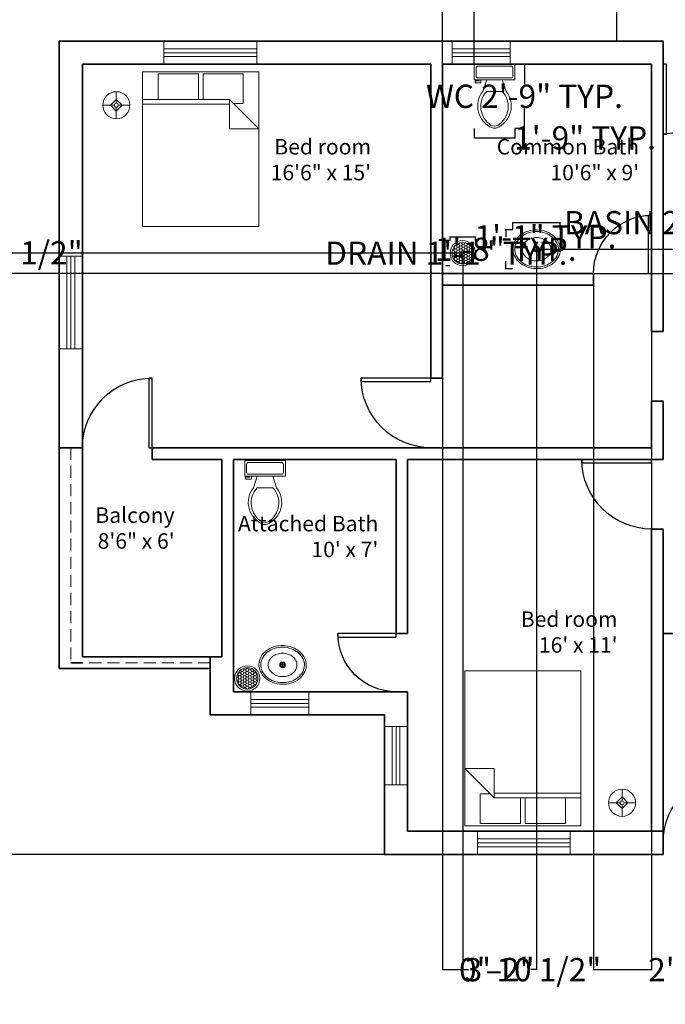
# Model space of a CAD drawing. Units: inches. Extents: x 2450 to 4494, y 1482 to 2597.
# Tile 4 of 7: x 3238 to 3571, y 1482 to 1990. Entities that reach past the tile are written whole.
import ezdxf

# ---------------------------------------------------------------- set-up
doc = ezdxf.new("R2010")
doc.units = ezdxf.units.IN
doc.header["$LTSCALE"] = 5
doc.header["$MEASUREMENT"] = 0
doc.linetypes.add('HIDDEN', pattern=[0.375, 0.25, -0.125])
for name, color, linetype, lineweight in [('A-ANNO-DIMS', 2, 'Continuous', 18), ('A-AREA-IDEN', 7, 'Continuous', 18), ('A-DOOR', 4, 'Continuous', 25), ('A-FLOR-EDGE', 7, 'Continuous', 25), ('A-FLOR-FIXT', 9, 'Continuous', 18), ('A-FURN', 8, 'Continuous', 18), ('A-GLAZ', 4, 'Continuous', 18), ('A-WALL', 7, 'Continuous', 35), ('A-WALL-HIDN', 7, 'HIDDEN', 18)]:
    doc.layers.add(name, color=color, linetype=linetype, lineweight=lineweight)
doc.styles.get("Standard").update_dxf_attribs({"font": 'arial.ttf'})
doc.dimstyles.get("Standard").update_dxf_attribs({"dimtxt": 12, "dimasz": 0.18, "dimexe": 0.18, "dimexo": 0.0625, "dimgap": 0.09, "dimtad": 0, "dimtih": 1, "dimtoh": 1, "dimdec": 0, "dimzin": 0, "dimdsep": 46, "dimlunit": 3, "dimtxsty": 'Standard', "dimcen": 0.09, "dimadec": 0, "dimazin": 0, "dimtfac": 1, "dimtdec": 0, "dimtofl": 0, "dimtmove": 0, "dimatfit": 3, "dimfxl": 1, "dimtolj": 1, "dimtzin": 0, "dimarcsym": 0})

# ---------------------------------------------------------------- blocks, each defined once
blk = doc.blocks.new('*U2')
for p, q in [((0, 0), (0, -6)), ((36, 0), (36, -6))]:
    blk.add_line(p, q)
blk.add_lwpolyline([(0, 0), (0, 36), (1.75, 36), (1.75, 0)], close=True)
blk.add_arc((0, 0), 36, 0, 90)
blk = doc.blocks.new('*U3')
for p, q in [((0, 0), (0, -6)), ((30, 0), (30, -6))]:
    blk.add_line(p, q)
blk.add_lwpolyline([(0, 0), (0, 30), (1.75, 30), (1.75, 0)], close=True)
blk.add_arc((0, 0), 30, 0, 90)
blk = doc.blocks.new('*U5')
for p, q in [((-36, 0), (-36, 6)), ((0, 0), (0, 6))]:
    blk.add_line(p, q)
blk.add_lwpolyline([(0, 0), (0, -36), (-1.75, -36), (-1.75, 0)], close=True)
blk.add_arc((0, 0), 36, 180, 270)
blk = doc.blocks.new('Bed - Queen')
for p, q in [((0, -80.00003), (0, 0)), ((0, 0), (59.99999, 0)), ((59.99999, 0), (59.99999, -80.00003)), ((7.99999, -1.2), (28.79998, -1.2)), ((7.99999, -14.4), (7.99999, -1.2)), ((28.79998, -1.2), (28.79998, -14.4)), ((31.19999, -1.2), (51.99999, -1.2)), ((31.19999, -14.4), (31.19999, -1.2)), ((51.99999, -1.2), (51.99999, -16.4)), ((0, -14.4), (44.8, -14.4)), ((59.99999, -29.6), (44.8, -14.4)), ((44.8, -14.4), (44.8, -29.6)), ((44.8, -16.8), (0, -16.8)), ((51.99999, -16.4), (46.79936, -16.4)), ((44.8, -29.6), (59.99999, -29.6)), ((59.99999, -80.00003), (0, -80.00003))]:
    blk.add_line(p, q)
blk = doc.blocks.new('Lamp - Table')
for p, q in [((0, 7), (0, 1)), ((-1, 0), (-7, 0)), ((0, 3), (-3, 0)), ((-3, 0), (0, -3)), ((3, 0), (0, 3)), ((0, -3), (3, 0)), ((1, 0), (7, 0)), ((0, -1), (0, -7))]:
    blk.add_line(p, q)
for radius in [7, 1]:
    blk.add_circle((0, 0), radius)
blk = doc.blocks.new('Toilet - top')
for p, q in [((9.5, -6), (9.5, -2)), ((-10, -8.5), (-8, -8.5)), ((-10, -9.5), (-10, -8.5)), ((-7, -9.5), (-10, -9.5)), ((-8, -8.5), (-8, -8)), ((-7, -8), (-7, -9.5)), ((-4, -8), (-6, -14)), ((4, -8), (6, -14)), ((4, -14), (-4, -14))]:
    blk.add_line(p, q)
blk.add_lwpolyline([(10.5, -8), (10.5, 0), (-10.5, 0), (-10.5, -8)], close=True)
for points in [[(-9.5, -2), (-9.5, -6)], [(8.5, -1), (-8.5, -1)], [(-8.5, -7), (8.5, -7)]]:
    blk.add_lwpolyline(points)
for centre, radius, start, end in [((-8.62, -1.88), 0.884, 81.8699, 188.1301), ((8.62, -1.88), 0.884, 351.8699, 98.1301), ((-8.62, -6.12), 0.884, 171.8699, 278.1301), ((8.62, -6.12), 0.884, 261.8699, 8.1301), ((3.52, -21.58), 12.17, 141.4691, 247.9714), ((4.2, -21.82), 11.33, 136.3677, 238.9468), ((-3.52, -21.58), 12.17, 292.0284, 38.5307), ((-4.2, -21.82), 11.33, 301.053, 43.6321), ((0, -27.88), 4, 245.7318, 294.2682), ((0, -29), 4, 254.8605, 285.1395)]:
    blk.add_arc(centre, radius, start, end)
blk = doc.blocks.new('Sink - Oval top')
for p, q in [((-1, 0), (1, 0)), ((0, 1), (0, -1))]:
    blk.add_line(p, q)
for points in [[(-12.23, 0.39, 0.117634), (-11.46, -3.36, 0.104469), (-8.88, -6.8, 0.090016), (-5.08, -9.07, 0.08192), (-0.32, -10.02, 0.08192), (4.49, -9.38, 0.090016), (8.42, -7.36, 0.104469), (11.22, -4.09, 0.117634), (12.23, -0.39, 0.117634), (11.46, 3.36, 0.104469), (8.88, 6.8, 0.090016), (5.08, 9.07, 0.08192), (0.32, 10.02, 0.08192), (-4.49, 9.38, 0.090016), (-8.42, 7.36, 0.104469), (-11.22, 4.09, 0.117634)], [(-11.29, 0.16, 0.118622), (-10.52, -3.25, 0.104678), (-8.07, -6.36, 0.089562), (-4.54, -8.37, 0.081185), (-0.13, -9.15, 0.081185), (4.3, -8.49, 0.089562), (7.89, -6.58, 0.104678), (10.42, -3.55, 0.118622), (11.29, -0.16, 0.118622), (10.52, 3.25, 0.104678), (8.07, 6.36, 0.089562), (4.54, 8.37, 0.081185), (0.13, 9.15, 0.081185), (-4.3, 8.49, 0.089562), (-7.89, 6.58, 0.104678), (-10.42, 3.55, 0.118622)], [(-7.42, 0.08, 0.118283), (-6.91, -2.17, 0.104607), (-5.29, -4.21, 0.089718), (-2.97, -5.53, 0.081436), (-0.07, -6.04, 0.081436), (2.84, -5.59, 0.089718), (5.2, -4.33, 0.104607), (6.86, -2.32, 0.118283), (7.42, -0.08, 0.118283), (6.91, 2.17, 0.104607), (5.29, 4.21, 0.089718), (2.97, 5.53, 0.081436), (0.07, 6.04, 0.081436), (-2.84, 5.59, 0.089718), (-5.2, 4.33, 0.104607), (-6.86, 2.32, 0.118283)]]:
    blk.add_lwpolyline(points, format="xyb", close=True)
for radius in [1.5, 1]:
    blk.add_circle((0, 0), radius)
blk = doc.blocks.new('WIN-30-FRAME')
for p, q in [((0, 0), (0, 12)), ((0, 12), (30, 12)), ((30, 12), (30, 0)), ((30, 8), (0, 8)), ((30, 6), (0, 6)), ((30, 4), (0, 4)), ((30, 0), (0, 0))]:
    blk.add_line(p, q)
blk = doc.blocks.new('WIN-48-FRAME')
for p, q in [((48, 12), (0, 12)), ((0, 12), (0, 0)), ((48, 0), (48, 12)), ((48, 8), (0, 8)), ((48, 6), (0, 6)), ((48, 4), (0, 4)), ((0, 0), (48, 0))]:
    blk.add_line(p, q)
blk = doc.blocks.new('WIN-30-PART-FRAME')
for p, q in [((12, 30), (0, 30)), ((0, 30), (0, 0)), ((4, 30), (4, 0)), ((6, 30), (6, 0)), ((8, 30), (8, 0)), ((12, 6), (12, 30)), ((0, 0), (12, 0))]:
    blk.add_line(p, q)
blk = doc.blocks.new('WIN-48-PART-FRAME')
for p, q in [((48, 12), (0, 12)), ((0, 12), (0, 0)), ((48, 0), (48, 12)), ((48, 8), (0, 8)), ((48, 6), (0, 6)), ((48, 4), (0, 4)), ((24, 0), (48, 0))]:
    blk.add_line(p, q)
blk = doc.blocks.new('WIN-48-OPEN-SIDE')
for p, q in [((0, 48), (12, 48)), ((4, 48), (4, 0)), ((6, 48), (6, 0)), ((8, 48), (8, 0)), ((12, 48), (12, 0)), ((12, 0), (0, 0))]:
    blk.add_line(p, q)
blk = doc.blocks.new('DRAIN-FLOOR-ROUND')
at = {"ltscale": 5}
h = blk.add_hatch(dxfattribs=at)
h.set_pattern_fill('HONEY', color=256, scale=7)
h.set_pattern_definition([(0, (-4161.689, -1861.538), (1.3125, 0.75777223), [0.875, -1.75]), (120, (-4161.689, -1861.538), (-1.3125, 0.75777223), [0.875, -1.75]), (60, (-4161.689, -1861.538), (3e-16, 1.51554446), [-1.75, 0.875])])
h.paths.add_polyline_path([(1, 6.52, 1), (12.03, 6.52, 1)])
for radius in [6.52, 5.52]:
    blk.add_circle((6.52, 6.52), radius, dxfattribs=at)
blk = doc.blocks.new('*D53')
at = {"layer": 'A-ANNO-DIMS', "color": 0, "lineweight": -2, "ltscale": 5, "transparency": 16777216}
for p, q in [((3493.72, 1967.27), (3498.8, 1967.27)), ((3498.62, 1967.09), (3498.62, 1957.04)), ((3498.62, 1934.4), (3498.62, 1944.45)), ((3493.72, 1934.22), (3498.8, 1934.22))]:
    blk.add_line(p, q, dxfattribs=at)
at = {"layer": 'A-ANNO-DIMS', "color": 0, "ltscale": 5, "transparency": 16777216}
for points in [[(3498.59, 1967.09), (3498.65, 1967.09), (3498.62, 1967.27)], [(3498.59, 1934.4), (3498.65, 1934.4), (3498.62, 1934.22)]]:
    blk.add_solid(points, dxfattribs=at)
at = {"layer": 'Defpoints', "color": 0, "ltscale": 5, "transparency": 16777216}
for p in [(3493.66, 1967.27), (3498.62, 1967.27), (3493.66, 1934.22)]:
    blk.add_point(p, dxfattribs=at)
at = {"layer": 'A-ANNO-DIMS', "color": 0, "ltscale": 5, "transparency": 16777216, "insert": (3498.62, 1950.74), "char_height": 12, "attachment_point": 5}
blk.add_mtext('\\A1;WC 2\'-9" TYP.', dxfattribs=at)
blk = doc.blocks.new('*D54')
at = {"layer": 'A-ANNO-DIMS', "color": 0, "lineweight": -2, "ltscale": 5, "transparency": 16777216}
for p, q in [((3472.66, 1934.16), (3472.66, 1929.08)), ((3493.66, 1934.16), (3493.66, 1929.08)), ((3472.84, 1929.26), (3493.48, 1929.26)), ((3493.66, 1929.26), (3493.84, 1929.26))]:
    blk.add_line(p, q, dxfattribs=at)
at = {"layer": 'A-ANNO-DIMS', "color": 0, "ltscale": 5, "transparency": 16777216}
for points in [[(3472.84, 1929.29), (3472.84, 1929.23), (3472.66, 1929.26)], [(3493.48, 1929.29), (3493.48, 1929.23), (3493.66, 1929.26)]]:
    blk.add_solid(points, dxfattribs=at)
at = {"layer": 'Defpoints', "color": 0, "ltscale": 5, "transparency": 16777216}
for p in [(3472.66, 1934.22), (3493.66, 1934.22), (3493.66, 1929.26)]:
    blk.add_point(p, dxfattribs=at)
at = {"layer": 'A-ANNO-DIMS', "color": 0, "ltscale": 5, "transparency": 16777216, "insert": (3529.94, 1929.26), "char_height": 12, "attachment_point": 5}
blk.add_mtext('\\A1;1\'-9" TYP.', dxfattribs=at)
blk = doc.blocks.new('*D55')
at = {"layer": 'A-ANNO-DIMS', "color": 0, "lineweight": -2, "ltscale": 5, "transparency": 16777216}
for p, q in [((3492.61, 1881.89), (3492.61, 1885.69)), ((3492.79, 1885.51), (3516.98, 1885.51)), ((3517.16, 1881.89), (3517.16, 1885.69)), ((3517.16, 1885.51), (3517.34, 1885.51))]:
    blk.add_line(p, q, dxfattribs=at)
at = {"layer": 'A-ANNO-DIMS', "color": 0, "ltscale": 5, "transparency": 16777216}
for points in [[(3492.79, 1885.54), (3492.79, 1885.48), (3492.61, 1885.51)], [(3516.98, 1885.54), (3516.98, 1885.48), (3517.16, 1885.51)]]:
    blk.add_solid(points, dxfattribs=at)
at = {"layer": 'Defpoints', "color": 0, "ltscale": 5, "transparency": 16777216}
for p in [(3492.61, 1881.83), (3517.16, 1885.51), (3517.16, 1881.83)]:
    blk.add_point(p, dxfattribs=at)
at = {"layer": 'A-ANNO-DIMS', "color": 0, "ltscale": 5, "transparency": 16777216, "insert": (3595.2, 1885.51), "char_height": 12, "attachment_point": 5}
blk.add_mtext('\\A1;BASIN 2\'-0 1/2" TYP.', dxfattribs=at)
blk = doc.blocks.new('*D56')
at = {"layer": 'A-ANNO-DIMS', "color": 0, "lineweight": -2, "ltscale": 5, "transparency": 16777216}
for p, q in [((3492.55, 1881.83), (3488.75, 1881.83)), ((3488.93, 1881.65), (3488.93, 1877.98)), ((3492.55, 1861.7), (3488.75, 1861.7)), ((3488.93, 1861.88), (3488.93, 1865.55))]:
    blk.add_line(p, q, dxfattribs=at)
at = {"layer": 'A-ANNO-DIMS', "color": 0, "ltscale": 5, "transparency": 16777216}
for points in [[(3488.9, 1881.65), (3488.96, 1881.65), (3488.93, 1881.83)], [(3488.9, 1861.88), (3488.96, 1861.88), (3488.93, 1861.7)]]:
    blk.add_solid(points, dxfattribs=at)
at = {"layer": 'Defpoints', "color": 0, "ltscale": 5, "transparency": 16777216}
for p in [(3488.93, 1881.83), (3492.61, 1881.83), (3492.61, 1861.7)]:
    blk.add_point(p, dxfattribs=at)
at = {"layer": 'A-ANNO-DIMS', "color": 0, "ltscale": 5, "transparency": 16777216, "insert": (3488.93, 1871.76), "char_height": 12, "attachment_point": 5}
blk.add_mtext('\\A1;1\'-8" TYP.', dxfattribs=at)
blk = doc.blocks.new('*D57')
at = {"layer": 'A-ANNO-DIMS', "color": 0, "lineweight": -2, "ltscale": 5, "transparency": 16777216}
for p, q in [((3460.16, 1876.24), (3458.09, 1876.24)), ((3458.27, 1876.06), (3458.27, 1875.84)), ((3460.16, 1863.21), (3458.09, 1863.21)), ((3458.27, 1863.39), (3458.27, 1863.6))]:
    blk.add_line(p, q, dxfattribs=at)
at = {"layer": 'A-ANNO-DIMS', "color": 0, "ltscale": 5, "transparency": 16777216}
for points in [[(3458.24, 1876.06), (3458.3, 1876.06), (3458.27, 1876.24)], [(3458.24, 1863.39), (3458.3, 1863.39), (3458.27, 1863.21)]]:
    blk.add_solid(points, dxfattribs=at)
at = {"layer": 'Defpoints', "color": 0, "ltscale": 5, "transparency": 16777216}
for p in [(3458.27, 1876.24), (3460.22, 1876.24), (3460.22, 1863.21)]:
    blk.add_point(p, dxfattribs=at)
at = {"layer": 'A-ANNO-DIMS', "color": 0, "ltscale": 5, "transparency": 16777216, "insert": (3458.27, 1869.72), "char_height": 12, "attachment_point": 5}
blk.add_mtext('\\A1;DRAIN 1\'-1" TYP.', dxfattribs=at)
blk = doc.blocks.new('*D58')
at = {"layer": 'A-ANNO-DIMS', "color": 0, "lineweight": -2, "ltscale": 5, "transparency": 16777216}
for p, q in [((3460.22, 1876.3), (3460.22, 1878.37)), ((3460.4, 1878.19), (3473.08, 1878.19)), ((3473.26, 1876.3), (3473.26, 1878.37)), ((3473.26, 1878.19), (3473.44, 1878.19))]:
    blk.add_line(p, q, dxfattribs=at)
at = {"layer": 'A-ANNO-DIMS', "color": 0, "ltscale": 5, "transparency": 16777216}
for points in [[(3460.4, 1878.22), (3460.4, 1878.16), (3460.22, 1878.19)], [(3473.08, 1878.22), (3473.08, 1878.16), (3473.26, 1878.19)]]:
    blk.add_solid(points, dxfattribs=at)
at = {"layer": 'Defpoints', "color": 0, "ltscale": 5, "transparency": 16777216}
for p in [(3460.22, 1876.24), (3473.26, 1878.19), (3473.26, 1876.24)]:
    blk.add_point(p, dxfattribs=at)
at = {"layer": 'A-ANNO-DIMS', "color": 0, "ltscale": 5, "transparency": 16777216, "insert": (3509.53, 1878.19), "char_height": 12, "attachment_point": 5}
blk.add_mtext('\\A1;1\'-1" TYP.', dxfattribs=at)
blk = doc.blocks.new('*D72')
at = {"layer": 'A-ANNO-DIMS', "color": 0, "lineweight": -2, "ltscale": 5, "transparency": 16777216}
for p, q in [((3426.23, 2519.27), (3198.61, 2519.27)), ((3198.79, 2519.09), (3198.79, 2045.48)), ((3198.79, 1559.45), (3198.79, 2033.05)), ((3426.23, 1559.27), (3198.61, 1559.27))]:
    blk.add_line(p, q, dxfattribs=at)
at = {"layer": 'A-ANNO-DIMS', "color": 0, "ltscale": 5, "transparency": 16777216}
for points in [[(3198.76, 2519.09), (3198.82, 2519.09), (3198.79, 2519.27)], [(3198.76, 1559.45), (3198.82, 1559.45), (3198.79, 1559.27)]]:
    blk.add_solid(points, dxfattribs=at)
at = {"layer": 'Defpoints', "color": 0, "ltscale": 5, "transparency": 16777216}
for p in [(3198.79, 2519.27), (3426.29, 2519.27), (3426.29, 1559.27)]:
    blk.add_point(p, dxfattribs=at)
at = {"layer": 'A-ANNO-DIMS', "color": 0, "ltscale": 5, "transparency": 16777216, "insert": (3198.79, 2039.27), "char_height": 12, "attachment_point": 5}
blk.add_mtext('\\A1;80\'-0"', dxfattribs=at)
blk = doc.blocks.new('*D82')
at = {"layer": 'A-ANNO-DIMS', "color": 0, "lineweight": -2, "ltscale": 5, "transparency": 16777216}
for p, q in [((3456.29, 1967.33), (3456.29, 2578.95)), ((3456.47, 2578.77), (3472.48, 2578.77)), ((3472.66, 1967.33), (3472.66, 2578.95)), ((3472.66, 2578.77), (3472.84, 2578.77))]:
    blk.add_line(p, q, dxfattribs=at)
at = {"layer": 'A-ANNO-DIMS', "color": 0, "ltscale": 5, "transparency": 16777216}
for points in [[(3456.47, 2578.8), (3456.47, 2578.74), (3456.29, 2578.77)], [(3472.48, 2578.8), (3472.48, 2578.74), (3472.66, 2578.77)]]:
    blk.add_solid(points, dxfattribs=at)
at = {"layer": 'Defpoints', "color": 0, "ltscale": 5, "transparency": 16777216}
for p in [(3472.66, 2578.77), (3456.29, 1967.27), (3472.66, 1967.27)]:
    blk.add_point(p, dxfattribs=at)
at = {"layer": 'A-ANNO-DIMS', "color": 0, "ltscale": 5, "transparency": 16777216, "insert": (3502.3, 2578.77), "char_height": 12, "attachment_point": 5}
blk.add_mtext('\\A1;1\'-4 1/2"', dxfattribs=at)
blk = doc.blocks.new('*D83')
at = {"layer": 'A-ANNO-DIMS', "color": 0, "lineweight": -2, "ltscale": 5, "transparency": 16777216}
for p, q in [((3534.29, 1859.2), (3534.29, 1499.59)), ((3564.29, 1859.2), (3564.29, 1499.59)), ((3534.47, 1499.77), (3564.11, 1499.77)), ((3564.29, 1499.77), (3564.47, 1499.77))]:
    blk.add_line(p, q, dxfattribs=at)
at = {"layer": 'A-ANNO-DIMS', "color": 0, "ltscale": 5, "transparency": 16777216}
for points in [[(3534.47, 1499.8), (3534.47, 1499.74), (3534.29, 1499.77)], [(3564.11, 1499.8), (3564.11, 1499.74), (3564.29, 1499.77)]]:
    blk.add_solid(points, dxfattribs=at)
at = {"layer": 'Defpoints', "color": 0, "ltscale": 5, "transparency": 16777216}
for p in [(3534.29, 1859.27), (3564.29, 1859.27), (3564.29, 1499.77)]:
    blk.add_point(p, dxfattribs=at)
at = {"layer": 'A-ANNO-DIMS', "color": 0, "ltscale": 5, "transparency": 16777216, "insert": (3580.61, 1499.77), "char_height": 12, "attachment_point": 5}
blk.add_mtext('\\A1;2\'-6"', dxfattribs=at)
blk = doc.blocks.new('*D84')
at = {"layer": 'A-ANNO-DIMS', "color": 0, "lineweight": -2, "ltscale": 5, "transparency": 16777216}
for p, q in [((3466.74, 1869.66), (3466.74, 1499.59)), ((3456.29, 1859.2), (3456.29, 1499.59)), ((3456.47, 1499.77), (3466.56, 1499.77)), ((3466.74, 1499.77), (3466.92, 1499.77))]:
    blk.add_line(p, q, dxfattribs=at)
at = {"layer": 'A-ANNO-DIMS', "color": 0, "ltscale": 5, "transparency": 16777216}
for points in [[(3456.47, 1499.8), (3456.47, 1499.74), (3456.29, 1499.77)], [(3466.56, 1499.8), (3466.56, 1499.74), (3466.74, 1499.77)]]:
    blk.add_solid(points, dxfattribs=at)
at = {"layer": 'Defpoints', "color": 0, "ltscale": 5, "transparency": 16777216}
for p in [(3466.74, 1869.72), (3456.29, 1859.27), (3466.74, 1499.77)]:
    blk.add_point(p, dxfattribs=at)
at = {"layer": 'A-ANNO-DIMS', "color": 0, "ltscale": 5, "transparency": 16777216, "insert": (3501.6, 1499.77), "char_height": 12, "attachment_point": 5}
blk.add_mtext('\\A1;0\'-10 1/2"', dxfattribs=at)
blk = doc.blocks.new('*D85')
at = {"layer": 'A-ANNO-DIMS', "color": 0, "lineweight": -2, "ltscale": 5, "transparency": 16777216}
for p, q in [((3504.89, 1871.7), (3504.89, 1499.59)), ((3466.74, 1869.66), (3466.74, 1499.59)), ((3466.92, 1499.77), (3469.78, 1499.77)), ((3504.71, 1499.77), (3501.85, 1499.77))]:
    blk.add_line(p, q, dxfattribs=at)
at = {"layer": 'A-ANNO-DIMS', "color": 0, "ltscale": 5, "transparency": 16777216}
for points in [[(3466.92, 1499.8), (3466.92, 1499.74), (3466.74, 1499.77)], [(3504.71, 1499.8), (3504.71, 1499.74), (3504.89, 1499.77)]]:
    blk.add_solid(points, dxfattribs=at)
at = {"layer": 'Defpoints', "color": 0, "ltscale": 5, "transparency": 16777216}
for p in [(3504.89, 1871.76), (3466.74, 1869.72), (3504.89, 1499.77)]:
    blk.add_point(p, dxfattribs=at)
at = {"layer": 'A-ANNO-DIMS', "color": 0, "ltscale": 5, "transparency": 16777216, "insert": (3485.81, 1499.77), "char_height": 12, "attachment_point": 5}
blk.add_mtext('\\A1;3\'-2"', dxfattribs=at)
blk = doc.blocks.new('*D86')
at = {"layer": 'A-ANNO-DIMS', "color": 0, "lineweight": -2, "ltscale": 5, "transparency": 16777216}
for p, q in [((3466.68, 1869.72), (3198.61, 1869.72)), ((3198.79, 1869.72), (3198.79, 1869.9)), ((3198.79, 1869.9), (3198.97, 1869.9)), ((3198.79, 1859.45), (3198.79, 1869.54)), ((3456.23, 1859.27), (3198.61, 1859.27))]:
    blk.add_line(p, q, dxfattribs=at)
at = {"layer": 'A-ANNO-DIMS', "color": 0, "ltscale": 5, "transparency": 16777216}
for points in [[(3198.76, 1869.54), (3198.82, 1869.54), (3198.79, 1869.72)], [(3198.76, 1859.45), (3198.82, 1859.45), (3198.79, 1859.27)]]:
    blk.add_solid(points, dxfattribs=at)
at = {"layer": 'Defpoints', "color": 0, "ltscale": 5, "transparency": 16777216}
for p in [(3198.79, 1869.72), (3466.74, 1869.72), (3456.29, 1859.27)]:
    blk.add_point(p, dxfattribs=at)
at = {"layer": 'A-ANNO-DIMS', "color": 0, "ltscale": 5, "transparency": 16777216, "insert": (3233.65, 1869.9), "char_height": 12, "attachment_point": 5}
blk.add_mtext('\\A1;0\'-10 1/2"', dxfattribs=at)
blk = doc.blocks.new('*D87')
at = {"layer": 'A-ANNO-DIMS', "color": 0, "lineweight": -2, "ltscale": 5, "transparency": 16777216}
for p, q in [((3504.95, 1871.76), (4433.97, 1871.76)), ((4433.79, 1871.76), (4433.79, 1871.94)), ((4433.79, 1871.94), (4433.97, 1871.94)), ((4433.79, 1859.45), (4433.79, 1871.58)), ((3534.35, 1859.27), (4433.97, 1859.27))]:
    blk.add_line(p, q, dxfattribs=at)
at = {"layer": 'A-ANNO-DIMS', "color": 0, "ltscale": 5, "transparency": 16777216}
for points in [[(4433.76, 1871.58), (4433.82, 1871.58), (4433.79, 1871.76)], [(4433.76, 1859.45), (4433.82, 1859.45), (4433.79, 1859.27)]]:
    blk.add_solid(points, dxfattribs=at)
at = {"layer": 'Defpoints', "color": 0, "ltscale": 5, "transparency": 16777216}
for p in [(3504.89, 1871.76), (4433.79, 1871.76), (3534.29, 1859.27)]:
    blk.add_point(p, dxfattribs=at)
at = {"layer": 'A-ANNO-DIMS', "color": 0, "ltscale": 5, "transparency": 16777216, "insert": (4463.43, 1871.94), "char_height": 12, "attachment_point": 5}
blk.add_mtext('\\A1;1\'-0 1/2"', dxfattribs=at)

msp = doc.modelspace()

# ---------------------------------------------------------------- linework, layer by layer
at = {"layer": 'A-FLOR-EDGE', "ltscale": 5}
msp.add_line((3546.29, 1979.27), (3546.29, 2099.27), dxfattribs=at)
at = {"layer": 'A-WALL'}
for p, q in [((3258.29, 1655.27), (3258.29, 1979.27)), ((3258.29, 1979.27), (3570.29, 1979.27)), ((3570.29, 1967.27), (3570.29, 1979.27)), ((3270.29, 1769.27), (3270.29, 1967.27)), ((3270.29, 1967.27), (3450.29, 1967.27)), ((3450.29, 1967.27), (3450.29, 1805.27)), ((3456.29, 1967.27), (3564.29, 1967.27)), ((3456.29, 1967.27), (3456.29, 1805.27)), ((3564.29, 1967.27), (3564.29, 1859.27)), ((3570.29, 1967.27), (3570.29, 1829.27)), ((3456.29, 1859.27), (3534.29, 1859.27)), ((3534.29, 1859.27), (3534.29, 1853.27)), ((3564.29, 1859.27), (3564.29, 1853.27)), ((3456.29, 1853.27), (3534.29, 1853.27)), ((3564.29, 1853.27), (3564.29, 1829.27)), ((3564.29, 1829.27), (3570.29, 1829.27)), ((3456.29, 1805.27), (3450.29, 1805.27)), ((3564.29, 1793.27), (3564.29, 1769.27)), ((3564.29, 1793.27), (3570.29, 1793.27)), ((3570.29, 1793.27), (3570.29, 1763.27)), ((3270.29, 1769.27), (3258.29, 1769.27)), ((3270.29, 1769.27), (3270.29, 1763.27)), ((3306.29, 1769.27), (3450.29, 1769.27)), ((3306.29, 1769.27), (3306.29, 1763.27)), ((3456.29, 1769.27), (3450.29, 1769.27)), ((3456.29, 1769.27), (3564.29, 1769.27)), ((3270.29, 1661.27), (3270.29, 1763.27)), ((3306.29, 1763.27), (3342.29, 1763.27)), ((3342.29, 1661.27), (3342.29, 1763.27)), ((3348.29, 1643.27), (3348.29, 1763.27)), ((3348.29, 1763.27), (3432.29, 1763.27)), ((3432.29, 1673.27), (3432.29, 1763.27)), ((3438.29, 1673.27), (3438.29, 1763.27)), ((3438.29, 1763.27), (3450.29, 1763.27)), ((3450.29, 1763.27), (3456.29, 1763.27)), ((3456.29, 1763.27), (3564.29, 1763.27)), ((3564.29, 1763.27), (3570.29, 1763.27)), ((3564.29, 1727.27), (3564.29, 1571.27)), ((3564.29, 1727.27), (3570.29, 1727.27)), ((3570.29, 1727.27), (3570.29, 1571.27)), ((3432.29, 1673.27), (3438.29, 1673.27)), ((3570.29, 1673.27), (3702.29, 1673.27)), ((3270.29, 1658.27), (3264.29, 1658.27)), ((3270.29, 1661.27), (3342.29, 1661.27)), ((3336.29, 1655.27), (3336.29, 1661.27)), ((3270.29, 1655.27), (3258.29, 1655.27)), ((3270.29, 1655.27), (3336.29, 1655.27)), ((3336.29, 1631.27), (3336.29, 1655.27)), ((3348.29, 1643.27), (3432.29, 1643.27)), ((3432.29, 1643.27), (3438.29, 1643.27)), ((3438.29, 1571.27), (3438.29, 1643.27)), ((3348.29, 1631.27), (3336.29, 1631.27)), ((3348.29, 1631.27), (3426.29, 1631.27)), ((3426.29, 1571.27), (3426.29, 1631.27)), ((3426.29, 1571.27), (3426.29, 1559.27)), ((3570.29, 1571.27), (3438.29, 1571.27)), ((3570.29, 1571.27), (3570.29, 1559.27)), ((3570.29, 1559.27), (3426.29, 1559.27))]:
    msp.add_line(p, q, dxfattribs=at)
at = {"layer": 'A-WALL-HIDN', "ltscale": 5}
for p, q in [((3264.29, 1769.27), (3264.29, 1658.27)), ((3336.29, 1658.27), (3270.29, 1658.27))]:
    msp.add_line(p, q, dxfattribs=at)

# ---------------------------------------------------------------- block references
at = {"layer": 'A-DOOR', "xscale": -1}
for name, p in [('*U5', (3570.29, 1967.27)), ('*U3', (3564.29, 1859.27)), ('*U2', (3306.29, 1769.27)), ('*U2', (3606.29, 1565.27))]:
    msp.add_blockref(name, p, dxfattribs=at)
at = {"layer": 'A-DOOR', "xscale": -1, "rotation": 90}
for name, p in [('*U2', (3450.29, 1805.27)), ('*U2', (3564.29, 1763.27)), ('*U3', (3432.29, 1673.27))]:
    msp.add_blockref(name, p, dxfattribs=at)
at = {"layer": 'A-FLOR-FIXT', "ltscale": 5}
for name, p in [('Toilet - top', (3483.16, 1967.27)), ('Sink - Oval top', (3504.89, 1871.76)), ('Toilet - top', (3364.6, 1762.61)), ('Sink - Oval top', (3373.67, 1657.12))]:
    msp.add_blockref(name, p, dxfattribs=at)
at = {"layer": 'A-FLOR-FIXT'}
for p in [(3460.22, 1863.21), (3348.9, 1643.63)]:
    msp.add_blockref('DRAIN-FLOOR-ROUND', p, dxfattribs=at)
at = {"layer": 'A-FURN', "ltscale": 5}
for name, p in [('Bed - Queen', (3301.38, 1963.46)), ('Lamp - Table', (3287.78, 1946.13)), ('Lamp - Table', (3549.07, 1585.93))]:
    msp.add_blockref(name, p, dxfattribs=at)
at = {"layer": 'A-FURN', "ltscale": 5, "rotation": 180}
msp.add_blockref('Bed - Queen', (3527.77, 1574.1), dxfattribs=at)
at = {"layer": 'A-GLAZ', "rotation": 180}
for name, p in [('WIN-48-FRAME', (3360.29, 1979.27)), ('WIN-48-OPEN-SIDE', (3270.29, 1868.27)), ('WIN-30-FRAME', (3387.29, 1643.27))]:
    msp.add_blockref(name, p, dxfattribs=at)
at = {"layer": 'A-GLAZ'}
msp.add_blockref('WIN-30-FRAME', (3461.3, 1967.27), dxfattribs=at)
at = {"layer": 'A-GLAZ', "extrusion": (0, 0, -1), "zscale": -1}
for name, p in [('WIN-30-PART-FRAME', (-3438.29, 1595.27)), ('WIN-48-PART-FRAME', (-3522.29, 1559.27))]:
    msp.add_blockref(name, p, dxfattribs=at)

# ---------------------------------------------------------------- texts
at = {"layer": 'A-AREA-IDEN', "char_height": 8, "attachment_point": 3}
for s, insert in [('Bed room\\P16\'6" x 15\'', (3419.39, 1928.7)), ('Common Bath\\P10\'6" x 9\'', (3557.86, 1928.7)), ('Balcony\\P8\'6" x 6\'', (3317.89, 1738.45)), ("Attached Bath\\P10' x 7'", (3423.15, 1734.1)), ("Bed room\\P16' x 11'", (3546.72, 1684.77))]:
    msp.add_mtext_dynamic_manual_height_columns(s, width=155.5618, gutter_width=1, heights=[0], dxfattribs=dict(at, insert=insert))

# ---------------------------------------------------------------- dimensions: what is measured, and where the dimension line sits
at = {"layer": 'A-ANNO-DIMS', "ltscale": 5}
for base, p1, p2, picture, middle in [((3472.66, 2578.77), (3456.29, 1967.27), (3472.66, 1967.27), '*D82', (3502.3, 2578.77)), ((3504.8862, 1499.7657), (3466.7402, 1869.7226), (3504.8862, 1871.7639), '*D85', (3485.8132, 1499.7657)), ((3466.7402, 1499.7657), (3456.2899, 1859.2657), (3466.7402, 1869.7226), '*D84', (3501.6023, 1499.7657)), ((3564.29, 1499.77), (3534.29, 1859.27), (3564.29, 1859.27), '*D83', (3580.61, 1499.77))]:
    dim = msp.add_linear_dim(base=base, p1=p1, p2=p2, dimstyle='Standard', override={"dimdec": 1, "dimlfac": 1, "dimrnd": 0, "dimzin": 1, "dimdsep": 46, "dimlunit": 4, "dimfrac": 2}, dxfattribs=at)
    dim.commit()
    dim.dimension.update_dxf_attribs({"geometry": picture, "text_midpoint": middle})
for base, p1, p2, picture, middle in [((3198.79, 2519.27), (3426.29, 1559.27), (3426.29, 2519.27), '*D72', (3198.79, 2039.27)), ((3198.7899, 1869.7226), (3456.2899, 1859.2657), (3466.7402, 1869.7226), '*D86', (3233.652, 1869.9026)), ((4433.79, 1871.76), (3534.29, 1859.27), (3504.89, 1871.76), '*D87', (4463.43, 1871.94))]:
    dim = msp.add_linear_dim(base=base, p1=p1, p2=p2, angle=90, dimstyle='Standard', override={"dimdec": 1, "dimlfac": 1, "dimrnd": 0, "dimzin": 1, "dimdsep": 46, "dimlunit": 4, "dimfrac": 2}, dxfattribs=at)
    dim.commit()
    dim.dimension.update_dxf_attribs({"geometry": picture, "text_midpoint": middle})
for base, p1, p2, text, picture, middle in [((3498.6182, 1967.2657), (3493.6612, 1934.2195), (3493.6612, 1967.2657), 'WC <> TYP.', '*D53', (3498.6182, 1950.7426)), ((3458.27, 1876.24), (3460.22, 1863.21), (3460.22, 1876.24), 'DRAIN <> TYP.', '*D57', (3458.27, 1869.72)), ((3488.93, 1881.83), (3492.61, 1861.7), (3492.61, 1881.83), '<> TYP.', '*D56', (3488.93, 1871.76))]:
    dim = msp.add_linear_dim(base=base, p1=p1, p2=p2, angle=90, text=text, dimstyle='Standard', override={"dimdec": 1, "dimlfac": 1, "dimrnd": 0, "dimzin": 1, "dimdsep": 46, "dimlunit": 4, "dimfrac": 2}, dxfattribs=at)
    dim.commit()
    dim.dimension.update_dxf_attribs({"geometry": picture, "text_midpoint": middle})
for base, p1, p2, text, picture, middle in [((3493.66, 1929.26), (3472.66, 1934.22), (3493.66, 1934.22), '<> TYP.', '*D54', (3529.94, 1929.26)), ((3517.1616, 1885.5149), (3492.6107, 1881.8322), (3517.1616, 1881.8322), 'BASIN <> TYP.', '*D55', (3595.2024, 1885.5149)), ((3473.26, 1878.19), (3460.22, 1876.24), (3473.26, 1876.24), '<> TYP.', '*D58', (3509.53, 1878.19))]:
    dim = msp.add_linear_dim(base=base, p1=p1, p2=p2, text=text, dimstyle='Standard', override={"dimdec": 1, "dimlfac": 1, "dimrnd": 0, "dimzin": 1, "dimdsep": 46, "dimlunit": 4, "dimfrac": 2}, dxfattribs=at)
    dim.commit()
    dim.dimension.update_dxf_attribs({"geometry": picture, "text_midpoint": middle})

doc.saveas('drawing.dxf')
